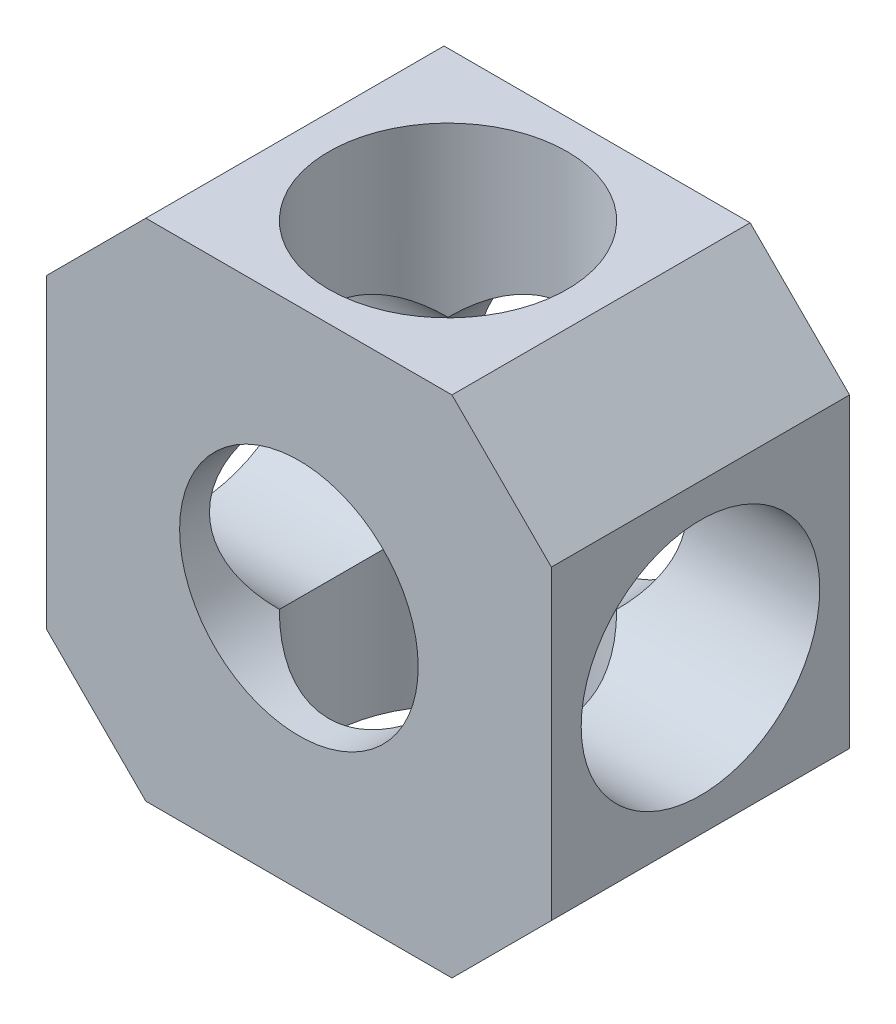
SolidWorks part; units mm, degrees
material "Plain Carbon Steel"
ref_plane "Front Plane" through (0, 0, 0) normal (0, 0, 1) x (1, 0, 0)
ref_plane "Top Plane" through (0, 0, 0) normal (0, 1, 0) x (1, 0, 0)
ref_plane "Right Plane" through (0, 0, 0) normal (1, 0, 0) x (0, 0, -1)
sketch "Nut Body Profile" plane through (0, 0, 0) normal (0, 0, 1) x (1, 0, 0)
  line L1 (-12.7, -12.7) -> (12.7, -12.7)
  line L2 (-12.7, -12.7) -> (-12.7, 12.7)
  line L3 (-12.7, 12.7) -> (12.7, 12.7)
  line L4 (12.7, -12.7) -> (12.7, 12.7)
  line L5 (-12.7, -12.7) -> (12.7, 12.7) construction
  line L6 (-12.7, 12.7) -> (12.7, -12.7) construction
  point P0 (0, 0)
  dimension "D1" = 25.4
  dimension "D2" = 25.4
extrude "Nut Body" add sketch "Nut Body Profile" along normal mid plane 15
chamfer "Edge Chamfers 5mm" distance 5 4 edges at (12.7, 12.7, 0) (-12.7, 12.7, 0) (-12.7, -12.7, 0) (12.7, -12.7, 0)
sketch "Axial Bore Profile" plane through (0, 0, -7.5) normal (0, 0, -1) x (-1, 0, 0)
  circle A0 centre (0, 0) radius 6
  dimension "D1" = 12
extrude "Axial Bore Ø12" cut sketch "Axial Bore Profile" against normal blind 15
sketch "Cross Bore A Profile" plane through (-12.7, 0, 0) normal (-1, 0, 0) x (0, 0, 1)
  circle A0 centre (0, 0) radius 6
  dimension "D1" = 12
extrude "Cross Bore A Ø12" cut sketch "Cross Bore A Profile" against normal through all
sketch "Cross Bore B Profile" plane through (0, 12.7, 0) normal (0, 1, 0) x (1, 0, 0)
  circle A0 centre (0, 0) radius 6
  dimension "D1" = 12
extrude "Cross Bore B Ø12" cut sketch "Cross Bore B Profile" against normal through all
